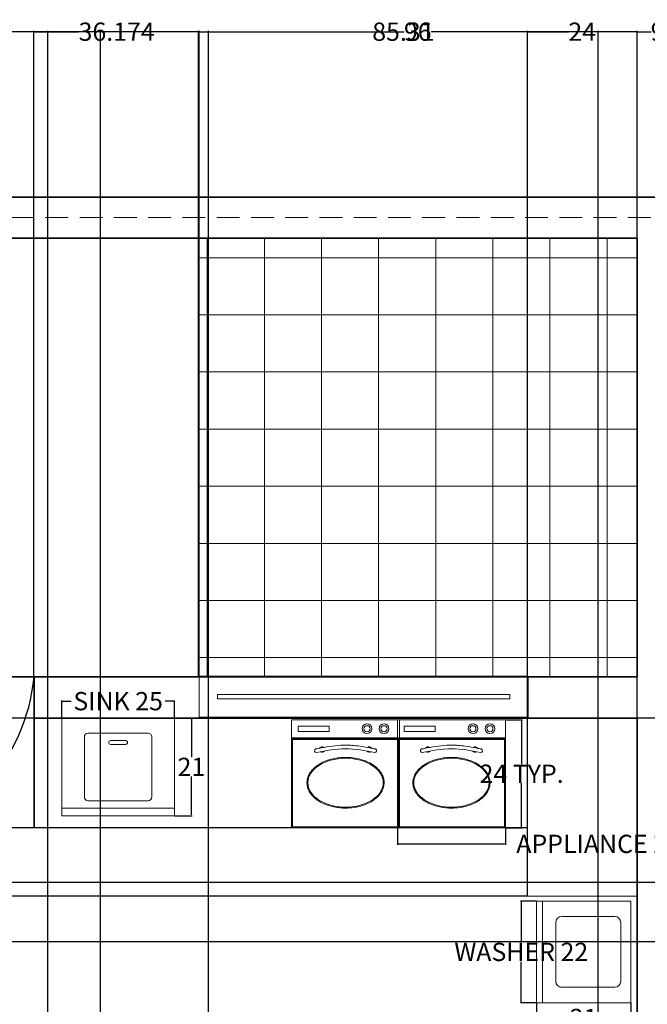
# Model space of a CAD drawing. Units: inches. Extents: x 1291 to 2095, y 532 to 1090.
# Tile 11 of 14: x 1559 to 1696, y 874 to 1090. Entities that reach past the tile are written whole.
import ezdxf

# ---------------------------------------------------------------- set-up
doc = ezdxf.new("R2010")
doc.units = ezdxf.units.IN
doc.header["$MEASUREMENT"] = 0
doc.linetypes.add('HIDDEN', pattern=[0.375, 0.25, -0.125])
for name, color, linetype, lineweight in [('A-ANNO-DIMS', 2, 'Continuous', 18), ('A-DOOR', 3, 'Continuous', 25), ('A-EQPM', 9, 'Continuous', 18), ('A-FLOR-CASE', 9, 'Continuous', 18), ('A-FLOR-FIXT', 9, 'Continuous', 18), ('A-FLOR-PATT', 252, 'Continuous', 13), ('A-GLAZ', 4, 'Continuous', 18), ('A-WALL', 7, 'Continuous', 35), ('A-WALL-HIDN', 8, 'HIDDEN', 13)]:
    doc.layers.add(name, color=color, linetype=linetype, lineweight=lineweight)
doc.styles.get("Standard").update_dxf_attribs({"font": 'arial.ttf'})
doc.dimstyles.get("Standard").update_dxf_attribs({"dimtxt": 4, "dimasz": 0.18, "dimexe": 0.18, "dimexo": 0.0625, "dimgap": 0.09, "dimtad": 0, "dimtih": 1, "dimtoh": 1, "dimdec": 0, "dimrnd": 6, "dimzin": 0, "dimdsep": 46, "dimlunit": 3, "dimtxsty": 'Standard', "dimcen": 0.09, "dimadec": 0, "dimazin": 0, "dimtfac": 1, "dimtdec": 0, "dimtofl": 0, "dimtmove": 0, "dimatfit": 3, "dimfxl": 1, "dimtolj": 1, "dimtzin": 0, "dimarcsym": 0})

# ---------------------------------------------------------------- blocks, each defined once
blk = doc.blocks.new('LAVAD-01')
for p, q in [((-0.3221, 0.3585), (-0.3221, -0.3915)), ((0.3279, 0.3585), (-0.3221, 0.3585)), ((-0.2721, 0.3585), (-0.2721, -0.3915)), ((0.3279, -0.3915), (0.3279, 0.3585)), ((0.2029, 0.2085), (-0.1971, 0.2085)), ((-0.2221, 0.1835), (-0.2221, -0.2165)), ((0.2279, -0.2165), (0.2279, 0.1835)), ((0.1529, 0.0335), (0.1529, -0.0665)), ((0.1654, 0.046), (0.1654, 0.046)), ((0.1779, -0.0665), (0.1779, 0.0335)), ((0.1654, -0.079), (0.1654, -0.079)), ((-0.1971, -0.2415), (0.2029, -0.2415)), ((-0.3221, -0.3915), (0.3279, -0.3915))]:
    blk.add_line(p, q)
for centre, radius, start, end in [((-0.1971, 0.1835), 0.025, 90, 180), ((0.2029, 0.1835), 0.025, 0, 90), ((0.1654, 0.0335), 0.0125, 90, 180), ((0.1654, 0.0335), 0.0125, 0, 90), ((0.1654, -0.0665), 0.0125, 180, 270), ((0.1654, -0.0665), 0.0125, 270, 360), ((-0.1971, -0.2165), 0.025, 180, 270), ((0.2029, -0.2165), 0.025, 270, 360)]:
    blk.add_arc(centre, radius, start, end)
blk = doc.blocks.new('LAVADORA')
for p, q in [((-0.35, 0.65), (-0.35, 0)), ((-0.35, 0.65), (0.35, 0.65)), ((0.35, 0.65), (0.35, 0)), ((-0.2031, 0.5795), (0.2031, 0.5795)), ((-0.2437, 0.5389), (-0.2437, 0.1732)), ((0.2437, 0.5389), (0.2437, 0.1732)), ((-0.2031, 0.1326), (0.2031, 0.1326)), ((-0.35, 0.0406), (0.35, 0.0406)), ((-0.35, 0), (0.35, 0))]:
    blk.add_line(p, q)
for centre, start, end in [((-0.2031, 0.5389), 90, 180), ((0.2031, 0.5389), 0, 90), ((-0.2031, 0.1732), 180, 270), ((0.2031, 0.1732), 270, 0)]:
    blk.add_arc(centre, 0.0406, start, end)
blk = doc.blocks.new('A$C7E884C79')
for p, q in [((0, 0), (0, 600)), ((0, 600), (0, 0)), ((0, 600), (600, 600)), ((600, 600), (600, 0)), ((600, 0), (600, 600)), ((600, 600), (600, 450)), ((600, 600), (600, 500)), ((600, 500), (0, 500)), ((600, 495), (0, 495)), ((600, 500), (600, 0)), ((0, 0), (600, 0))]:
    blk.add_line(p, q)
for points in [[(36.4, 564.7), (208.9, 564.7), (208.9, 535.3), (36.4, 535.3)], [(5, 490), (595, 490), (595, 5), (5, 5)]]:
    blk.add_lwpolyline(points, close=True)
for centre, radius in [((419.3, 550), 27), ((419.3, 550), 17), ((513.9, 550), 27), ((513.9, 550), 17)]:
    blk.add_circle(centre, radius)
for centre, radius, start, end in [((168.5, 434.2), 15, 50.7888, 150.367), ((431.5, 434.2), 15, 29.633, 129.2112), ((137.2, 428), 10, 107.9829, 276.9581), ((168.5, 434.2), 15, 234.0165, 327.1412), ((431.5, 434.2), 15, 212.8588, 305.9835), ((462.8, 428), 10, 263.0419, 72.0171)]:
    blk.add_arc(centre, radius, start, end)
blk.add_ellipse((300, 250), major_axis=(-209.5, 0), ratio=0.648352)
for points, knots in [([(134.1, 437.5), (144.6, 439.5), (155.1, 441.6), (186, 447.3), (206.5, 450.9), (247.9, 456.4), (268.7, 458.3), (293.5, 458.9), (297.3, 458.9), (304.8, 458.9), (308.5, 458.8), (319.7, 458.5), (327.1, 458.1), (349.4, 456.5), (364.1, 454.9), (399.8, 449.9), (420.6, 446.2), (449.5, 440.7), (457.7, 439.1), (465.9, 437.5)], [0, 0, 0, 0, 31.638865, 31.638865, 92.600143, 92.600143, 153.561421, 153.561421, 164.367647, 164.367647, 175.173874, 175.173874, 196.786327, 196.786327, 240.011233, 240.011233, 302.099201, 302.099201, 326.773065, 326.773065, 326.773065, 326.773065]), ([(85.5, 250), (85.5, 244.8), (85.9, 239.6), (88, 226.9), (90.2, 219.4), (96.4, 204.8), (100.4, 197.7), (109.9, 184.1), (115.6, 177.5), (128.3, 165.1), (135.4, 159.2), (150.9, 148.3), (159.3, 143.3), (177.1, 134.2), (186.6, 130.1), (206.5, 123), (216.8, 119.9), (238.1, 114.9), (249, 113), (271.2, 110.2), (282.5, 109.4), (305, 109), (316.4, 109.4), (338.8, 111.3), (349.8, 112.8), (371.5, 117), (382.1, 119.6), (402.5, 126), (412.3, 129.7), (431, 138.1), (439.8, 142.8), (456.2, 153), (463.8, 158.6), (477.6, 170.5), (483.8, 176.8), (494.6, 190.1), (499.2, 197), (506.7, 211.3), (509.5, 218.7), (513.4, 233.6), (514.4, 241.3), (514.6, 256.5), (513.8, 264.1), (510.2, 279.1), (507.6, 286.6), (500.4, 300.9), (496, 307.9), (485.5, 321.3), (479.5, 327.7), (466, 339.7), (458.5, 345.3), (442.4, 355.8), (433.6, 360.5), (415.2, 369.1), (405.5, 373), (385.2, 379.5), (374.7, 382.3), (353.1, 386.7), (342, 388.3), (319.7, 390.5), (308.4, 390.9), (285.8, 390.7), (274.5, 390.1), (252.3, 387.5), (241.3, 385.7), (219.9, 380.9), (209.5, 378), (189.5, 371), (179.9, 367.1), (161.8, 358.1), (153.3, 353.2), (137.6, 342.5), (130.3, 336.7), (117.3, 324.4), (111.6, 317.9), (101.6, 304.3), (97.5, 297.3), (91, 282.8), (88.6, 275.3), (86, 261.9), (85.5, 255.9), (85.5, 250)], [0, 0, 0, 0, 0.108301, 0.108301, 0.267534, 0.267534, 0.426768, 0.426768, 0.586002, 0.586002, 0.745235, 0.745235, 0.904469, 0.904469, 1.063703, 1.063703, 1.222936, 1.222936, 1.38217, 1.38217, 1.541404, 1.541404, 1.700637, 1.700637, 1.859871, 1.859871, 2.019105, 2.019105, 2.178339, 2.178339, 2.337572, 2.337572, 2.496806, 2.496806, 2.65604, 2.65604, 2.815273, 2.815273, 2.974507, 2.974507, 3.133741, 3.133741, 3.292974, 3.292974, 3.452208, 3.452208, 3.611442, 3.611442, 3.770676, 3.770676, 3.929909, 3.929909, 4.089143, 4.089143, 4.248377, 4.248377, 4.40761, 4.40761, 4.566844, 4.566844, 4.726078, 4.726078, 4.885311, 4.885311, 5.044545, 5.044545, 5.203779, 5.203779, 5.363012, 5.363012, 5.522246, 5.522246, 5.68148, 5.68148, 5.840714, 5.840714, 5.999947, 5.999947, 6.159181, 6.159181, 6.283185, 6.283185, 6.283185, 6.283185])]:
    blk.add_open_spline(points, degree=3, knots=knots)
blk.add_open_spline([(138, 417.8), (192, 428.4), (300, 449.4), (408, 428.4), (462, 417.8)], degree=3)
blk = doc.blocks.new('WIN-72IN')
for points in [[(0, 0), (0, 9), (72, 9), (72, 0)], [(4, 4), (4, 5), (68, 5), (68, 4)]]:
    blk.add_lwpolyline(points, close=True)
blk = doc.blocks.new('*D16')
at = {"layer": 'A-ANNO-DIMS', "color": 0, "lineweight": -2, "transparency": 16777216}
for p, q in [((1672.02, 896.73), (1668.56, 896.73)), ((1668.74, 896.55), (1668.74, 887.76)), ((1668.74, 874.66), (1668.74, 883.44)), ((1672.02, 874.48), (1668.56, 874.48))]:
    blk.add_line(p, q, dxfattribs=at)
at = {"layer": 'A-ANNO-DIMS', "color": 0, "transparency": 16777216}
for points in [[(1668.71, 896.55), (1668.77, 896.55), (1668.74, 896.73)], [(1668.71, 874.66), (1668.77, 874.66), (1668.74, 874.48)]]:
    blk.add_solid(points, dxfattribs=at)
at = {"layer": 'Defpoints', "color": 0, "transparency": 16777216}
for p in [(1672.08, 896.73), (1668.74, 874.48), (1672.08, 874.48)]:
    blk.add_point(p, dxfattribs=at)
at = {"layer": 'A-ANNO-DIMS', "color": 0, "transparency": 16777216, "insert": (1668.74, 885.6), "char_height": 4, "attachment_point": 5}
blk.add_mtext('\\A1;WASHER 22', dxfattribs=at)
blk = doc.blocks.new('*D17')
at = {"layer": 'A-ANNO-DIMS', "color": 0, "lineweight": -2, "transparency": 16777216}
for p, q in [((1672.08, 874.42), (1672.08, 870.96)), ((1692.74, 874.42), (1692.74, 870.96)), ((1672.26, 871.14), (1679.81, 871.14)), ((1692.56, 871.14), (1685.01, 871.14))]:
    blk.add_line(p, q, dxfattribs=at)
at = {"layer": 'A-ANNO-DIMS', "color": 0, "transparency": 16777216}
for points in [[(1672.26, 871.17), (1672.26, 871.11), (1672.08, 871.14)], [(1692.56, 871.17), (1692.56, 871.11), (1692.74, 871.14)]]:
    blk.add_solid(points, dxfattribs=at)
at = {"layer": 'Defpoints', "color": 0, "transparency": 16777216}
for p in [(1672.08, 874.48), (1692.74, 874.48), (1692.74, 871.14)]:
    blk.add_point(p, dxfattribs=at)
at = {"layer": 'A-ANNO-DIMS', "color": 0, "transparency": 16777216, "insert": (1682.41, 871.14), "char_height": 4, "attachment_point": 5}
blk.add_mtext('\\A1;21', dxfattribs=at)
blk = doc.blocks.new('*D20')
at = {"layer": 'A-ANNO-DIMS', "color": 0, "lineweight": -2, "transparency": 16777216}
for p, q in [((1641.64, 912.72), (1641.64, 909.06)), ((1665.26, 912.72), (1665.26, 909.06)), ((1641.82, 909.24), (1665.08, 909.24)), ((1665.26, 909.24), (1665.44, 909.24))]:
    blk.add_line(p, q, dxfattribs=at)
at = {"layer": 'A-ANNO-DIMS', "color": 0, "transparency": 16777216}
for points in [[(1641.82, 909.27), (1641.82, 909.21), (1641.64, 909.24)], [(1665.08, 909.27), (1665.08, 909.21), (1665.26, 909.24)]]:
    blk.add_solid(points, dxfattribs=at)
at = {"layer": 'Defpoints', "color": 0, "transparency": 16777216}
for p in [(1641.64, 912.78), (1665.26, 912.78), (1665.26, 909.24)]:
    blk.add_point(p, dxfattribs=at)
at = {"layer": 'A-ANNO-DIMS', "color": 0, "transparency": 16777216, "insert": (1691.84, 909.24), "char_height": 4, "attachment_point": 5}
blk.add_mtext('\\A1;APPLIANCE 24 TYP.', dxfattribs=at)
blk = doc.blocks.new('*D21')
at = {"layer": 'A-ANNO-DIMS', "color": 0, "lineweight": -2, "transparency": 16777216}
for p, q in [((1665.33, 936.4), (1668.99, 936.4)), ((1668.81, 936.22), (1668.81, 926.69)), ((1668.81, 912.96), (1668.81, 922.49)), ((1665.33, 912.78), (1668.99, 912.78))]:
    blk.add_line(p, q, dxfattribs=at)
at = {"layer": 'A-ANNO-DIMS', "color": 0, "transparency": 16777216}
for points in [[(1668.78, 936.22), (1668.84, 936.22), (1668.81, 936.4)], [(1668.78, 912.96), (1668.84, 912.96), (1668.81, 912.78)]]:
    blk.add_solid(points, dxfattribs=at)
at = {"layer": 'Defpoints', "color": 0, "transparency": 16777216}
for p in [(1665.26, 936.4), (1668.81, 936.4), (1665.26, 912.78)]:
    blk.add_point(p, dxfattribs=at)
at = {"layer": 'A-ANNO-DIMS', "color": 0, "transparency": 16777216, "insert": (1668.81, 924.59), "char_height": 4, "attachment_point": 5}
blk.add_mtext('\\A1;24 TYP.', dxfattribs=at)
blk = doc.blocks.new('*D28')
at = {"layer": 'A-ANNO-DIMS', "color": 0, "lineweight": -2, "transparency": 16777216}
for p, q in [((1568.16, 936.84), (1568.16, 940.65)), ((1568.34, 940.47), (1570.23, 940.47)), ((1592.64, 940.47), (1590.75, 940.47)), ((1592.82, 936.84), (1592.82, 940.65))]:
    blk.add_line(p, q, dxfattribs=at)
at = {"layer": 'A-ANNO-DIMS', "color": 0, "transparency": 16777216}
for points in [[(1568.34, 940.5), (1568.34, 940.44), (1568.16, 940.47)], [(1592.64, 940.5), (1592.64, 940.44), (1592.82, 940.47)]]:
    blk.add_solid(points, dxfattribs=at)
at = {"layer": 'Defpoints', "color": 0, "transparency": 16777216}
for p in [(1568.16, 940.47), (1568.16, 936.77), (1592.82, 936.77)]:
    blk.add_point(p, dxfattribs=at)
at = {"layer": 'A-ANNO-DIMS', "color": 0, "transparency": 16777216, "insert": (1580.49, 940.47), "char_height": 4, "attachment_point": 5}
blk.add_mtext('\\A1;SINK 25', dxfattribs=at)
blk = doc.blocks.new('*D29')
at = {"layer": 'A-ANNO-DIMS', "color": 0, "lineweight": -2, "transparency": 16777216}
for p, q in [((1592.89, 936.77), (1596.7, 936.77)), ((1596.52, 936.59), (1596.52, 928.18)), ((1596.52, 915.58), (1596.52, 923.99)), ((1592.89, 915.4), (1596.7, 915.4))]:
    blk.add_line(p, q, dxfattribs=at)
at = {"layer": 'A-ANNO-DIMS', "color": 0, "transparency": 16777216}
for points in [[(1596.49, 936.59), (1596.55, 936.59), (1596.52, 936.77)], [(1596.49, 915.58), (1596.55, 915.58), (1596.52, 915.4)]]:
    blk.add_solid(points, dxfattribs=at)
at = {"layer": 'Defpoints', "color": 0, "transparency": 16777216}
for p in [(1592.82, 936.77), (1596.52, 936.77), (1592.82, 915.4)]:
    blk.add_point(p, dxfattribs=at)
at = {"layer": 'A-ANNO-DIMS', "color": 0, "transparency": 16777216, "insert": (1596.52, 926.09), "char_height": 4, "attachment_point": 5}
blk.add_mtext('\\A1;21', dxfattribs=at)
blk = doc.blocks.new('*D38')
at = {"layer": 'A-ANNO-DIMS', "color": 0, "lineweight": -2, "transparency": 16777216}
for p, q in [((1343.07, 1041.84), (1343.07, 1087.16)), ((1343.25, 1086.98), (1466.02, 1086.98)), ((1597.89, 1086.98), (1475.13, 1086.98)), ((1598.07, 1041.84), (1598.07, 1087.16))]:
    blk.add_line(p, q, dxfattribs=at)
at = {"layer": 'A-ANNO-DIMS', "color": 0, "transparency": 16777216}
for points in [[(1343.25, 1087.01), (1343.25, 1086.95), (1343.07, 1086.98)], [(1597.89, 1087.01), (1597.89, 1086.95), (1598.07, 1086.98)]]:
    blk.add_solid(points, dxfattribs=at)
at = {"layer": 'Defpoints', "color": 0, "transparency": 16777216}
for p in [(1598.07, 1086.98), (1343.07, 1041.78), (1598.07, 1041.78)]:
    blk.add_point(p, dxfattribs=at)
at = {"layer": 'A-ANNO-DIMS', "color": 0, "transparency": 16777216, "insert": (1470.57, 1086.98), "char_height": 4, "attachment_point": 5}
blk.add_mtext('\\A1;255', dxfattribs=at)
blk = doc.blocks.new('*D39')
at = {"layer": 'A-ANNO-DIMS', "color": 0, "lineweight": -2, "transparency": 16777216}
for p, q in [((1598.07, 1041.84), (1598.07, 1087.16)), ((1598.25, 1086.98), (1643.12, 1086.98)), ((1693.89, 1086.98), (1649.03, 1086.98)), ((1694.07, 1041.84), (1694.07, 1087.16))]:
    blk.add_line(p, q, dxfattribs=at)
at = {"layer": 'A-ANNO-DIMS', "color": 0, "transparency": 16777216}
for points in [[(1598.25, 1087.01), (1598.25, 1086.95), (1598.07, 1086.98)], [(1693.89, 1087.01), (1693.89, 1086.95), (1694.07, 1086.98)]]:
    blk.add_solid(points, dxfattribs=at)
at = {"layer": 'Defpoints', "color": 0, "transparency": 16777216}
for p in [(1694.07, 1086.98), (1598.07, 1041.78), (1694.07, 1041.78)]:
    blk.add_point(p, dxfattribs=at)
at = {"layer": 'A-ANNO-DIMS', "color": 0, "transparency": 16777216, "insert": (1646.07, 1086.98), "char_height": 4, "attachment_point": 5}
blk.add_mtext('\\A1;96', dxfattribs=at)
blk = doc.blocks.new('*D40')
at = {"layer": 'A-ANNO-DIMS', "color": 0, "lineweight": -2, "transparency": 16777216}
for p, q in [((1694.07, 1041.84), (1694.07, 1087.16)), ((1694.25, 1086.98), (1697.17, 1086.98)), ((1702.89, 1086.98), (1699.98, 1086.98)), ((1703.07, 1041.84), (1703.07, 1087.16))]:
    blk.add_line(p, q, dxfattribs=at)
at = {"layer": 'A-ANNO-DIMS', "color": 0, "transparency": 16777216}
for points in [[(1694.25, 1087.01), (1694.25, 1086.95), (1694.07, 1086.98)], [(1702.89, 1087.01), (1702.89, 1086.95), (1703.07, 1086.98)]]:
    blk.add_solid(points, dxfattribs=at)
at = {"layer": 'Defpoints', "color": 0, "transparency": 16777216}
for p in [(1703.07, 1086.98), (1694.07, 1041.78), (1703.07, 1041.78)]:
    blk.add_point(p, dxfattribs=at)
at = {"layer": 'A-ANNO-DIMS', "color": 0, "transparency": 16777216, "insert": (1698.57, 1086.98), "char_height": 4, "attachment_point": 5}
blk.add_mtext('\\A1;9', dxfattribs=at)
blk = doc.blocks.new('*D44')
at = {"layer": 'A-ANNO-DIMS', "color": 0, "lineweight": -2, "transparency": 16777216}
for p, q in [((1343.07, 579.84), (1343.07, 1087.16)), ((1343.25, 1086.98), (1451.42, 1086.98)), ((1576.43, 1086.98), (1468.26, 1086.98)), ((1576.61, 579.84), (1576.61, 1087.16))]:
    blk.add_line(p, q, dxfattribs=at)
at = {"layer": 'A-ANNO-DIMS', "color": 0, "transparency": 16777216}
for points in [[(1343.25, 1087.01), (1343.25, 1086.95), (1343.07, 1086.98)], [(1576.43, 1087.01), (1576.43, 1086.95), (1576.61, 1086.98)]]:
    blk.add_solid(points, dxfattribs=at)
at = {"layer": 'Defpoints', "color": 0, "transparency": 16777216}
for p in [(1576.61, 1086.98), (1343.07, 579.78), (1576.61, 579.78)]:
    blk.add_point(p, dxfattribs=at)
at = {"layer": 'A-ANNO-DIMS', "color": 0, "transparency": 16777216, "insert": (1459.84, 1086.98), "char_height": 4, "attachment_point": 5}
blk.add_mtext('\\A1;233.54', dxfattribs=at)
blk = doc.blocks.new('*D46')
at = {"layer": 'A-ANNO-DIMS', "color": 0, "lineweight": -2, "transparency": 16777216}
for p, q in [((1600.27, 579.84), (1600.27, 1087.16)), ((1600.45, 1086.98), (1636.47, 1086.98)), ((1685.4, 1086.98), (1649.38, 1086.98)), ((1685.58, 579.84), (1685.58, 1087.16))]:
    blk.add_line(p, q, dxfattribs=at)
at = {"layer": 'A-ANNO-DIMS', "color": 0, "transparency": 16777216}
for points in [[(1600.45, 1087.01), (1600.45, 1086.95), (1600.27, 1086.98)], [(1685.4, 1087.01), (1685.4, 1086.95), (1685.58, 1086.98)]]:
    blk.add_solid(points, dxfattribs=at)
at = {"layer": 'Defpoints', "color": 0, "transparency": 16777216}
for p in [(1685.58, 1086.98), (1600.27, 579.78), (1685.58, 579.78)]:
    blk.add_point(p, dxfattribs=at)
at = {"layer": 'A-ANNO-DIMS', "color": 0, "transparency": 16777216, "insert": (1642.93, 1086.98), "char_height": 4, "attachment_point": 5}
blk.add_mtext('\\A1;85.31', dxfattribs=at)
blk = doc.blocks.new('*D56')
at = {"layer": 'A-ANNO-DIMS', "color": 0, "lineweight": -2, "transparency": 16777216}
for p, q in [((1868.01, 936.78), (1297.69, 936.78)), ((1297.87, 936.6), (1297.87, 914.41)), ((1297.87, 887.96), (1297.87, 910.15)), ((1868.01, 887.78), (1297.69, 887.78))]:
    blk.add_line(p, q, dxfattribs=at)
at = {"layer": 'A-ANNO-DIMS', "color": 0, "transparency": 16777216}
for points in [[(1297.84, 936.6), (1297.9, 936.6), (1297.87, 936.78)], [(1297.84, 887.96), (1297.9, 887.96), (1297.87, 887.78)]]:
    blk.add_solid(points, dxfattribs=at)
at = {"layer": 'Defpoints', "color": 0, "transparency": 16777216}
for p in [(1297.87, 936.78), (1868.07, 936.78), (1868.07, 887.78)]:
    blk.add_point(p, dxfattribs=at)
at = {"layer": 'A-ANNO-DIMS', "color": 0, "transparency": 16777216, "insert": (1297.87, 912.28), "char_height": 4, "attachment_point": 5}
blk.add_mtext('\\A1;49', dxfattribs=at)
blk = doc.blocks.new('*D57')
at = {"layer": 'A-ANNO-DIMS', "color": 0, "lineweight": -2, "transparency": 16777216}
for p, q in [((1973.01, 900.78), (1297.69, 900.78)), ((1297.87, 900.6), (1297.87, 896.41)), ((1297.87, 887.96), (1297.87, 892.15)), ((1973.01, 887.78), (1297.69, 887.78))]:
    blk.add_line(p, q, dxfattribs=at)
at = {"layer": 'A-ANNO-DIMS', "color": 0, "transparency": 16777216}
for points in [[(1297.84, 900.6), (1297.9, 900.6), (1297.87, 900.78)], [(1297.84, 887.96), (1297.9, 887.96), (1297.87, 887.78)]]:
    blk.add_solid(points, dxfattribs=at)
at = {"layer": 'Defpoints', "color": 0, "transparency": 16777216}
for p in [(1297.87, 900.78), (1973.07, 900.78), (1973.07, 887.78)]:
    blk.add_point(p, dxfattribs=at)
at = {"layer": 'A-ANNO-DIMS', "color": 0, "transparency": 16777216, "insert": (1297.87, 894.28), "char_height": 4, "attachment_point": 5}
blk.add_mtext('\\A1;13', dxfattribs=at)
blk = doc.blocks.new('*D59')
at = {"layer": 'A-ANNO-DIMS', "color": 0, "lineweight": -2, "transparency": 16777216}
for p, q in [((2009.01, 900.78), (1297.69, 900.78)), ((1297.87, 900.6), (1297.87, 877.91)), ((1297.87, 850.96), (1297.87, 873.65)), ((2009.01, 850.78), (1297.69, 850.78))]:
    blk.add_line(p, q, dxfattribs=at)
at = {"layer": 'A-ANNO-DIMS', "color": 0, "transparency": 16777216}
for points in [[(1297.84, 900.6), (1297.9, 900.6), (1297.87, 900.78)], [(1297.84, 850.96), (1297.9, 850.96), (1297.87, 850.78)]]:
    blk.add_solid(points, dxfattribs=at)
at = {"layer": 'Defpoints', "color": 0, "transparency": 16777216}
for p in [(1297.87, 900.78), (2009.07, 900.78), (2009.07, 850.78)]:
    blk.add_point(p, dxfattribs=at)
at = {"layer": 'A-ANNO-DIMS', "color": 0, "transparency": 16777216, "insert": (1297.87, 875.78), "char_height": 4, "attachment_point": 5}
blk.add_mtext('\\A1;50', dxfattribs=at)
blk = doc.blocks.new('*D63')
at = {"layer": 'A-ANNO-DIMS', "color": 0, "lineweight": -2, "transparency": 16777216}
for p, q in [((1529.07, 723.84), (1529.07, 1087.16)), ((1529.25, 1086.98), (1544.12, 1086.98)), ((1564.89, 1086.98), (1550.03, 1086.98)), ((1565.07, 723.84), (1565.07, 1087.16))]:
    blk.add_line(p, q, dxfattribs=at)
at = {"layer": 'A-ANNO-DIMS', "color": 0, "transparency": 16777216}
for points in [[(1529.25, 1087.01), (1529.25, 1086.95), (1529.07, 1086.98)], [(1564.89, 1087.01), (1564.89, 1086.95), (1565.07, 1086.98)]]:
    blk.add_solid(points, dxfattribs=at)
at = {"layer": 'Defpoints', "color": 0, "transparency": 16777216}
for p in [(1565.07, 1086.98), (1529.07, 723.78), (1565.07, 723.78)]:
    blk.add_point(p, dxfattribs=at)
at = {"layer": 'A-ANNO-DIMS', "color": 0, "transparency": 16777216, "insert": (1547.07, 1086.98), "char_height": 4, "attachment_point": 5}
blk.add_mtext('\\A1;36', dxfattribs=at)
blk = doc.blocks.new('*D71')
at = {"layer": 'A-ANNO-DIMS', "color": 0, "lineweight": -2, "transparency": 16777216}
for p, q in [((1526.07, 945.84), (1526.07, 1087.16)), ((1526.25, 1086.98), (1541.12, 1086.98)), ((1561.89, 1086.98), (1547.03, 1086.98)), ((1562.07, 945.84), (1562.07, 1087.16))]:
    blk.add_line(p, q, dxfattribs=at)
at = {"layer": 'A-ANNO-DIMS', "color": 0, "transparency": 16777216}
for points in [[(1526.25, 1087.01), (1526.25, 1086.95), (1526.07, 1086.98)], [(1561.89, 1087.01), (1561.89, 1086.95), (1562.07, 1086.98)]]:
    blk.add_solid(points, dxfattribs=at)
at = {"layer": 'Defpoints', "color": 0, "transparency": 16777216}
for p in [(1562.07, 1086.98), (1526.07, 945.78), (1562.07, 945.78)]:
    blk.add_point(p, dxfattribs=at)
at = {"layer": 'A-ANNO-DIMS', "color": 0, "transparency": 16777216, "insert": (1544.07, 1086.98), "char_height": 4, "attachment_point": 5}
blk.add_mtext('\\A1;36', dxfattribs=at)
blk = doc.blocks.new('*D72')
at = {"layer": 'A-ANNO-DIMS', "color": 0, "lineweight": -2, "transparency": 16777216}
for p, q in [((1562.07, 945.84), (1562.07, 1087.16)), ((1562.25, 1086.98), (1571.78, 1086.98)), ((1598.07, 1086.98), (1588.54, 1086.98)), ((1598.25, 946.01), (1598.25, 1087.16))]:
    blk.add_line(p, q, dxfattribs=at)
at = {"layer": 'A-ANNO-DIMS', "color": 0, "transparency": 16777216}
for points in [[(1562.25, 1087.01), (1562.25, 1086.95), (1562.07, 1086.98)], [(1598.07, 1087.01), (1598.07, 1086.95), (1598.25, 1086.98)]]:
    blk.add_solid(points, dxfattribs=at)
at = {"layer": 'Defpoints', "color": 0, "transparency": 16777216}
for p in [(1598.25, 1086.98), (1598.25, 945.95), (1562.07, 945.78)]:
    blk.add_point(p, dxfattribs=at)
at = {"layer": 'A-ANNO-DIMS', "color": 0, "transparency": 16777216, "insert": (1580.16, 1086.98), "char_height": 4, "attachment_point": 5}
blk.add_mtext('\\A1;36.174', dxfattribs=at)
blk = doc.blocks.new('*D78')
at = {"layer": 'A-ANNO-DIMS', "color": 0, "lineweight": -2, "transparency": 16777216}
for p, q in [((1562.01, 936.78), (1297.69, 936.78)), ((1297.87, 936.6), (1297.87, 926.88)), ((1297.87, 912.96), (1297.87, 922.68)), ((1562.01, 912.78), (1297.69, 912.78))]:
    blk.add_line(p, q, dxfattribs=at)
at = {"layer": 'A-ANNO-DIMS', "color": 0, "transparency": 16777216}
for points in [[(1297.84, 936.6), (1297.9, 936.6), (1297.87, 936.78)], [(1297.84, 912.96), (1297.9, 912.96), (1297.87, 912.78)]]:
    blk.add_solid(points, dxfattribs=at)
at = {"layer": 'Defpoints', "color": 0, "transparency": 16777216}
for p in [(1297.87, 936.78), (1562.07, 936.78), (1562.07, 912.78)]:
    blk.add_point(p, dxfattribs=at)
at = {"layer": 'A-ANNO-DIMS', "color": 0, "transparency": 16777216, "insert": (1297.87, 924.78), "char_height": 4, "attachment_point": 5}
blk.add_mtext('\\A1;24', dxfattribs=at)
blk = doc.blocks.new('*D79')
at = {"layer": 'A-ANNO-DIMS', "color": 0, "lineweight": -2, "transparency": 16777216}
for p, q in [((1670.07, 897.84), (1670.07, 1087.16)), ((1670.25, 1086.98), (1679.09, 1086.98)), ((1693.89, 1086.98), (1685.05, 1086.98)), ((1694.07, 897.84), (1694.07, 1087.16))]:
    blk.add_line(p, q, dxfattribs=at)
at = {"layer": 'A-ANNO-DIMS', "color": 0, "transparency": 16777216}
for points in [[(1670.25, 1087.01), (1670.25, 1086.95), (1670.07, 1086.98)], [(1693.89, 1087.01), (1693.89, 1086.95), (1694.07, 1086.98)]]:
    blk.add_solid(points, dxfattribs=at)
at = {"layer": 'Defpoints', "color": 0, "transparency": 16777216}
for p in [(1694.07, 1086.98), (1670.07, 897.78), (1694.07, 897.78)]:
    blk.add_point(p, dxfattribs=at)
at = {"layer": 'A-ANNO-DIMS', "color": 0, "transparency": 16777216, "insert": (1682.07, 1086.98), "char_height": 4, "attachment_point": 5}
blk.add_mtext('\\A1;24', dxfattribs=at)
blk = doc.blocks.new('*D80')
at = {"layer": 'A-ANNO-DIMS', "color": 0, "lineweight": -2, "transparency": 16777216}
for p, q in [((1670.01, 912.78), (1297.69, 912.78)), ((1297.87, 912.6), (1297.87, 907.41)), ((1297.87, 897.96), (1297.87, 903.15)), ((1670.01, 897.78), (1297.69, 897.78))]:
    blk.add_line(p, q, dxfattribs=at)
at = {"layer": 'A-ANNO-DIMS', "color": 0, "transparency": 16777216}
for points in [[(1297.84, 912.6), (1297.9, 912.6), (1297.87, 912.78)], [(1297.84, 897.96), (1297.9, 897.96), (1297.87, 897.78)]]:
    blk.add_solid(points, dxfattribs=at)
at = {"layer": 'Defpoints', "color": 0, "transparency": 16777216}
for p in [(1297.87, 912.78), (1670.07, 912.78), (1670.07, 897.78)]:
    blk.add_point(p, dxfattribs=at)
at = {"layer": 'A-ANNO-DIMS', "color": 0, "transparency": 16777216, "insert": (1297.87, 905.28), "char_height": 4, "attachment_point": 5}
blk.add_mtext('\\A1;15', dxfattribs=at)

msp = doc.modelspace()

# ---------------------------------------------------------------- hatches: boundary and pattern name
at = {"layer": 'A-FLOR-PATT'}
h = msp.add_hatch(dxfattribs=at)
h.set_pattern_fill('NET', color=256, scale=100)
h.paths.add_polyline_path([(1694.0735, 1041.7804), (1598.0735, 1041.7804), (1598.0735, 945.9453), (1670.2475, 945.9453), (1694.0735, 945.9242)])

# ---------------------------------------------------------------- linework, layer by layer
at = {"layer": 'A-DOOR'}
msp.add_arc((1521.8491, 949.5186), 40.3978, 280.290544, 354.690499, dxfattribs=at)
at = {"layer": 'A-FLOR-CASE'}
for p, q in [((1670.0735, 912.7804), (1562.0735, 912.7804)), ((1670.0735, 897.7804), (1670.0735, 912.7804)), ((1694.0735, 897.7804), (1670.0735, 897.7804))]:
    msp.add_line(p, q, dxfattribs=at)
at = {"layer": 'A-WALL'}
for p, q in [((2054.0735, 1050.7804), (1334.0735, 1050.7804)), ((1694.0735, 1041.7804), (1343.0735, 1041.7804)), ((1598.0735, 945.7804), (1598.0735, 1041.7804)), ((1694.0735, 945.7804), (1694.0735, 1041.7804)), ((1694.0735, 945.7804), (1526.0735, 945.7804)), ((1562.0735, 912.7804), (1562.0735, 945.7804)), ((1694.0735, 936.7804), (1562.0735, 936.7804)), ((1694.0735, 861.7804), (1694.0735, 936.7804))]:
    msp.add_line(p, q, dxfattribs=at)
at = {"layer": 'A-WALL-HIDN', "ltscale": 20}
msp.add_line((2049.5735, 1046.2804), (1338.5735, 1046.2804), dxfattribs=at)

# ---------------------------------------------------------------- block references
at = {"layer": 'A-EQPM', "xscale": 0.0393700787401575, "yscale": 0.0393700787401575, "zscale": 0.0393700787401575}
for p in [(1618.4553, 912.7804), (1641.6418, 912.7804)]:
    msp.add_blockref('A$C7E884C79', p, dxfattribs=at)
at = {"layer": 'A-EQPM', "xscale": 31.77820954593226, "yscale": 31.77820954593226, "zscale": 31.77820954593226, "rotation": 270}
msp.add_blockref('LAVADORA', (1672.0814, 885.6032), dxfattribs=at)
at = {"layer": 'A-FLOR-FIXT', "xscale": 32.88456246090828, "yscale": 32.88456246090828, "zscale": 32.88456246090828, "rotation": 90}
msp.add_blockref('LAVAD-01', (1579.948, 925.9895), dxfattribs=at)
at = {"layer": 'A-GLAZ'}
msp.add_blockref('WIN-72IN', (1598.2479, 936.9457), dxfattribs=at)

# ---------------------------------------------------------------- dimensions: what is measured, and where the dimension line sits
at = {"layer": 'A-ANNO-DIMS'}
for base, p1, p2, override, picture, middle in [((1598.0735, 1086.9804), (1343.0735, 1041.7804), (1598.0735, 1041.7804), {"dimdec": 0, "dimlfac": 1, "dimrnd": 0, "dimzin": 0, "dimdsep": 46, "dimlunit": 2}, '*D38', (1470.5735, 1086.9804)), ((1576.6107, 1086.9804), (1343.0735, 579.7804), (1576.6107, 579.7804), {"dimdec": 2, "dimlfac": 1, "dimrnd": 0, "dimzin": 0, "dimdsep": 46, "dimlunit": 2}, '*D44', (1459.8421, 1086.9804)), ((1562.0735, 1086.9804), (1526.0735, 945.7804), (1562.0735, 945.7804), {"dimdec": 0, "dimlfac": 1, "dimrnd": 0, "dimzin": 0, "dimdsep": 46, "dimlunit": 2}, '*D71', (1544.0735, 1086.9804)), ((1565.0735, 1086.9804), (1529.0735, 723.7804), (1565.0735, 723.7804), {"dimdec": 0, "dimlfac": 1, "dimrnd": 0, "dimzin": 0, "dimdsep": 46, "dimlunit": 2}, '*D63', (1547.0735, 1086.9804)), ((1598.2475, 1086.9804), (1562.0735, 945.7804), (1598.2475, 945.9453), {"dimdec": 3, "dimlfac": 1, "dimrnd": 0, "dimzin": 0, "dimdsep": 46, "dimlunit": 2}, '*D72', (1580.1605, 1086.9804)), ((1694.0735, 1086.9804), (1598.0735, 1041.7804), (1694.0735, 1041.7804), {"dimdec": 0, "dimlfac": 1, "dimrnd": 0, "dimzin": 0, "dimdsep": 46, "dimlunit": 2}, '*D39', (1646.0735, 1086.9804)), ((1685.5842, 1086.9804), (1600.2697, 579.7804), (1685.5842, 579.7804), {"dimdec": 2, "dimlfac": 1, "dimrnd": 0, "dimzin": 0, "dimdsep": 46, "dimlunit": 2}, '*D46', (1642.927, 1086.9804)), ((1694.0735, 1086.9804), (1670.0735, 897.7804), (1694.0735, 897.7804), {"dimdec": 0, "dimlfac": 1, "dimrnd": 0, "dimzin": 0, "dimdsep": 46, "dimlunit": 2}, '*D79', (1682.0735, 1086.9804)), ((1703.0735, 1086.9804), (1694.0735, 1041.7804), (1703.0735, 1041.7804), {"dimdec": 0, "dimlfac": 1, "dimrnd": 0, "dimzin": 0, "dimdsep": 46, "dimlunit": 2}, '*D40', (1698.5735, 1086.9804)), ((1692.7372, 871.1441), (1672.0814, 874.4808), (1692.7372, 874.4808), {"dimdec": 0, "dimlfac": 1, "dimrnd": 0, "dimzin": 0, "dimdsep": 46, "dimlunit": 2}, '*D17', (1682.4093, 871.1441))]:
    dim = msp.add_linear_dim(base=base, p1=p1, p2=p2, dimstyle='Standard', override=override, dxfattribs=at)
    dim.commit()
    dim.dimension.update_dxf_attribs({"geometry": picture, "text_midpoint": middle})
for base, p1, p2, angle, text, picture, middle in [((1568.1599, 940.473), (1592.8233, 936.7735), (1568.1599, 936.7735), 180, 'SINK <>', '*D28', (1580.4916, 940.473)), ((1668.8071, 936.4025), (1665.2638, 912.7804), (1665.2638, 936.4025), 90, '<> TYP.', '*D21', (1668.8071, 924.5914)), ((1668.7447, 874.4808), (1672.0814, 896.7256), (1672.0814, 874.4808), 270, 'WASHER <>', '*D16', (1668.7447, 885.6032))]:
    dim = msp.add_linear_dim(base=base, p1=p1, p2=p2, angle=angle, text=text, dimstyle='Standard', override={"dimdec": 0, "dimlfac": 1, "dimrnd": 0, "dimzin": 0, "dimdsep": 46, "dimlunit": 2}, dxfattribs=at)
    dim.commit()
    dim.dimension.update_dxf_attribs({"geometry": picture, "text_midpoint": middle})
for base, p1, p2, picture, middle in [((1297.8735, 936.7804), (1868.0735, 887.7804), (1868.0735, 936.7804), '*D56', (1297.8735, 912.2804)), ((1297.8735, 936.7804), (1562.0735, 912.7804), (1562.0735, 936.7804), '*D78', (1297.8735, 924.7804)), ((1596.5229, 936.7735), (1592.8233, 915.3985), (1592.8233, 936.7735), '*D29', (1596.5229, 926.086)), ((1297.8735, 912.7804), (1670.0735, 897.7804), (1670.0735, 912.7804), '*D80', (1297.8735, 905.2804)), ((1297.8735, 900.7804), (1973.0735, 887.7804), (1973.0735, 900.7804), '*D57', (1297.8735, 894.2804)), ((1297.8735, 900.7804), (2009.0735, 850.7804), (2009.0735, 900.7804), '*D59', (1297.8735, 875.7804))]:
    dim = msp.add_linear_dim(base=base, p1=p1, p2=p2, angle=90, dimstyle='Standard', override={"dimdec": 0, "dimlfac": 1, "dimrnd": 0, "dimzin": 0, "dimdsep": 46, "dimlunit": 2}, dxfattribs=at)
    dim.commit()
    dim.dimension.update_dxf_attribs({"geometry": picture, "text_midpoint": middle})
dim = msp.add_linear_dim(base=(1665.2638, 909.2371), p1=(1641.6418, 912.7804), p2=(1665.2638, 912.7804), text='APPLIANCE <> TYP.', dimstyle='Standard', override={"dimdec": 0, "dimlfac": 1, "dimrnd": 0, "dimzin": 0, "dimdsep": 46, "dimlunit": 2}, dxfattribs=at)
dim.commit()
dim.dimension.update_dxf_attribs({"geometry": '*D20', "text_midpoint": (1691.8449, 909.2371)})

doc.saveas('drawing.dxf')
